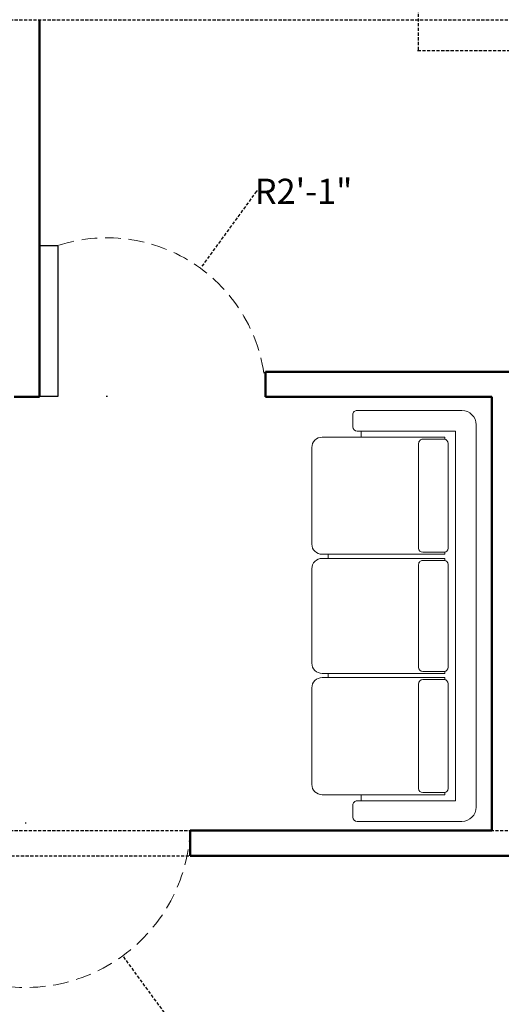
# Model space of a CAD drawing. Units: inches. Extents: x 513 to 1142, y 396 to 927.
# Tile 26 of 31: x 922 to 998, y 614 to 770. Entities that reach past the tile are written whole.
import ezdxf

# ---------------------------------------------------------------- set-up
doc = ezdxf.new("R2010")
doc.units = ezdxf.units.IN
doc.header["$MEASUREMENT"] = 0
doc.linetypes.add('DASHED', pattern=[0.75, 0.5, -0.25])
for name, color, linetype, lineweight in [('A-ANNO-DIMS', 2, 'DASHED', 18), ('A-DOOR', 4, 'Continuous', 25), ('A-DOOR-SWNG', 4, 'DASHED', 13), ('A-WALL', 7, 'Continuous', 50), ('furniture', 92, 'Continuous', 18)]:
    doc.layers.add(name, color=color, linetype=linetype, lineweight=lineweight)
doc.styles.get("Standard").update_dxf_attribs({"font": 'arial.ttf'})
doc.dimstyles.get("Standard").update_dxf_attribs({"dimtxt": 4, "dimasz": 0.18, "dimexe": 0.18, "dimexo": 0.0625, "dimgap": 0.09, "dimtad": 0, "dimtih": 1, "dimtoh": 1, "dimdec": 0, "dimrnd": 6, "dimzin": 0, "dimdsep": 46, "dimlunit": 3, "dimtxsty": 'Standard', "dimcen": 0.09, "dimadec": 0, "dimazin": 0, "dimtfac": 1, "dimtdec": 0, "dimtofl": 0, "dimtmove": 0, "dimatfit": 3, "dimfxl": 1, "dimtolj": 1, "dimtzin": 0, "dimarcsym": 0})

# ---------------------------------------------------------------- blocks, each defined once
blk = doc.blocks.new('A$C06FC73D7')
for p, q in [((1.93, 0.8), (0.07, 0.8)), ((0, 0.73), (0, 0.22)), ((2, 0.22), (2, 0.73)), ((0.1, 0.22), (0.1, 0.7)), ((0.1, 0.7), (1.9, 0.7)), ((1.9, 0.7), (1.9, 0.22)), ((0.13, 0.6479), (0.13, 0.05)), ((0.1404, 0.6479), (0.13, 0.6479)), ((0.14, 0.54), (0.14, 0.6437)), ((0.67, 0.6637), (0.16, 0.6637)), ((0.7, 0.6479), (0.6896, 0.6479)), ((0.69, 0.54), (0.69, 0.6437)), ((0.7, 0.05), (0.7, 0.6479)), ((0.72, 0.05), (0.72, 0.6479)), ((0.7304, 0.6479), (0.72, 0.6479)), ((0.73, 0.54), (0.73, 0.6437)), ((1.25, 0.6637), (0.75, 0.6637)), ((1.28, 0.6479), (1.2696, 0.6479)), ((1.27, 0.54), (1.27, 0.6437)), ((1.28, 0.05), (1.28, 0.6479)), ((1.3, 0.05), (1.3, 0.6479)), ((1.3104, 0.6479), (1.3, 0.6479)), ((1.31, 0.54), (1.31, 0.6437)), ((1.84, 0.6637), (1.33, 0.6637)), ((1.87, 0.6479), (1.86, 0.6479)), ((1.86, 0.54), (1.86, 0.6437)), ((1.87, 0.05), (1.87, 0.6479)), ((0.67, 0.52), (0.16, 0.52)), ((1.25, 0.52), (0.75, 0.52)), ((1.84, 0.52), (1.33, 0.52)), ((0.13, 0.24), (0.1, 0.24)), ((1.9, 0.24), (1.87, 0.24)), ((0.02, 0.2), (0.08, 0.2)), ((1.92, 0.2), (1.98, 0.2)), ((0.72, 0.08), (0.7, 0.08)), ((1.3, 0.08), (1.28, 0.08)), ((0.65, 0), (0.18, 0)), ((1.23, 0), (0.77, 0)), ((1.82, 0), (1.35, 0))]:
    blk.add_line(p, q)
for centre, radius, start, end in [((0.07, 0.73), 0.07, 90, 180), ((1.93, 0.73), 0.07, 0, 90), ((0.16, 0.6437), 0.02, 90, 180), ((0.67, 0.6437), 0.02, 0, 90), ((0.75, 0.6437), 0.02, 90, 180), ((1.25, 0.6437), 0.02, 0, 90), ((1.33, 0.6437), 0.02, 90, 180), ((1.84, 0.6437), 0.02, 0, 90), ((0.16, 0.54), 0.02, 180, 270), ((0.67, 0.54), 0.02, 270, 0), ((0.75, 0.54), 0.02, 180, 270), ((1.25, 0.54), 0.02, 270, 0), ((1.33, 0.54), 0.02, 180, 270), ((1.84, 0.54), 0.02, 270, 0), ((0.02, 0.22), 0.02, 180, 270), ((0.08, 0.22), 0.02, 270, 0), ((1.92, 0.22), 0.02, 180, 270), ((1.98, 0.22), 0.02, 270, 0), ((0.18, 0.05), 0.05, 180, 270), ((0.65, 0.05), 0.05, 270, 0), ((0.77, 0.05), 0.05, 180, 270), ((1.23, 0.05), 0.05, 270, 0), ((1.35, 0.05), 0.05, 180, 270), ((1.82, 0.05), 0.05, 270, 0)]:
    blk.add_arc(centre, radius, start, end)
blk = doc.blocks.new('A$C2BDD4447')
blk.add_blockref('A$C06FC73D7', (0, 0))
blk = doc.blocks.new('DOOR-LEAF-24IN')
blk.add_lwpolyline([(3, 24), (3, 0), (0, 0), (0, 24)], close=True)
blk = doc.blocks.new('*D117')
at = {"layer": 'A-ANNO-DIMS', "color": 0, "lineweight": -2, "transparency": 16777216}
for p, q in [((999.94, 862.98), (985.15, 862.98)), ((985.33, 862.8), (985.33, 816.24)), ((985.33, 765.36), (985.33, 811.92)), ((999.94, 765.18), (985.15, 765.18))]:
    blk.add_line(p, q, dxfattribs=at)
at = {"layer": 'A-ANNO-DIMS', "color": 0, "transparency": 16777216}
for points in [[(985.3, 862.8), (985.36, 862.8), (985.33, 862.98)], [(985.3, 765.36), (985.36, 765.36), (985.33, 765.18)]]:
    blk.add_solid(points, dxfattribs=at)
at = {"layer": 'Defpoints', "color": 0, "transparency": 16777216}
for p in [(1000, 862.98), (985.33, 765.18), (1000, 765.18)]:
    blk.add_point(p, dxfattribs=at)
at = {"layer": 'A-ANNO-DIMS', "color": 0, "transparency": 16777216, "insert": (985.33, 814.08), "char_height": 4, "attachment_point": 5}
blk.add_mtext('\\A1;BED GROUP 8\'-2" TYP.', dxfattribs=at)
blk = doc.blocks.new('*D149')
at = {"layer": 'A-ANNO-DIMS', "color": 0, "lineweight": -2, "transparency": 16777216}
for p, q in [((840.06, 770.16), (1131.58, 770.16)), ((1131.4, 769.98), (1131.4, 707.79)), ((1131.4, 641.34), (1131.4, 703.53)), ((840.06, 641.16), (1131.58, 641.16))]:
    blk.add_line(p, q, dxfattribs=at)
at = {"layer": 'A-ANNO-DIMS', "color": 0, "transparency": 16777216}
for points in [[(1131.37, 769.98), (1131.43, 769.98), (1131.4, 770.16)], [(1131.37, 641.34), (1131.43, 641.34), (1131.4, 641.16)]]:
    blk.add_solid(points, dxfattribs=at)
at = {"layer": 'Defpoints', "color": 0, "transparency": 16777216}
for p in [(840, 770.16), (1131.4, 770.16), (840, 641.16)]:
    blk.add_point(p, dxfattribs=at)
at = {"layer": 'A-ANNO-DIMS', "color": 0, "transparency": 16777216, "insert": (1131.4, 705.66), "char_height": 4, "attachment_point": 5}
blk.add_mtext('\\A1;10\'-9"', dxfattribs=at)
blk = doc.blocks.new('*D173')
at = {"layer": 'A-ANNO-DIMS', "color": 0, "lineweight": -2, "transparency": 16777216}
for p, q in [((904.06, 637.16), (1131.58, 637.16)), ((1131.4, 636.98), (1131.4, 618.76)), ((1131.4, 596.27), (1131.4, 614.49)), ((904.06, 596.09), (1131.58, 596.09))]:
    blk.add_line(p, q, dxfattribs=at)
at = {"layer": 'A-ANNO-DIMS', "color": 0, "transparency": 16777216}
for points in [[(1131.37, 636.98), (1131.43, 636.98), (1131.4, 637.16)], [(1131.37, 596.27), (1131.43, 596.27), (1131.4, 596.09)]]:
    blk.add_solid(points, dxfattribs=at)
at = {"layer": 'Defpoints', "color": 0, "transparency": 16777216}
for p in [(904, 637.16), (1131.4, 637.16), (904, 596.09)]:
    blk.add_point(p, dxfattribs=at)
at = {"layer": 'A-ANNO-DIMS', "color": 0, "transparency": 16777216, "insert": (1131.4, 616.63), "char_height": 4, "attachment_point": 5}
blk.add_mtext('\\A1;3\'-5"', dxfattribs=at)
blk = doc.blocks.new('*D180')
at = {"layer": 'A-ANNO-DIMS', "color": 0, "lineweight": -2, "transparency": 16777216}
for p, q in [((922.75, 642.37), (922.93, 642.37)), ((922.84, 642.28), (922.84, 642.46)), ((947.56, 608.55), (938.4, 621.09)), ((947.74, 608.55), (947.56, 608.55))]:
    blk.add_line(p, q, dxfattribs=at)
at = {"layer": 'A-ANNO-DIMS', "color": 0, "transparency": 16777216}
blk.add_solid([(938.42, 621.11), (938.37, 621.07), (938.29, 621.24)], dxfattribs=at)
at = {"layer": 'Defpoints', "color": 0, "transparency": 16777216}
for p in [(922.84, 642.37), (938.29, 621.24)]:
    blk.add_point(p, dxfattribs=at)
at = {"layer": 'A-ANNO-DIMS', "color": 0, "transparency": 16777216, "insert": (955.06, 608.55), "char_height": 4, "attachment_point": 5}
blk.add_mtext('\\A1;R2\'-2"', dxfattribs=at)
blk = doc.blocks.new('*D181')
at = {"layer": 'A-ANNO-DIMS', "color": 0, "lineweight": -2, "transparency": 16777216}
for p, q in [((959.54, 742.86), (950.73, 730.77)), ((959.72, 742.86), (959.54, 742.86)), ((935.67, 710.24), (935.85, 710.24)), ((935.76, 710.15), (935.76, 710.33))]:
    blk.add_line(p, q, dxfattribs=at)
at = {"layer": 'A-ANNO-DIMS', "color": 0, "transparency": 16777216}
blk.add_solid([(950.71, 730.79), (950.75, 730.76), (950.62, 730.63)], dxfattribs=at)
at = {"layer": 'Defpoints', "color": 0, "transparency": 16777216}
for p in [(950.62, 730.63), (935.76, 710.24)]:
    blk.add_point(p, dxfattribs=at)
at = {"layer": 'A-ANNO-DIMS', "color": 0, "transparency": 16777216, "insert": (967.04, 742.86), "char_height": 4, "attachment_point": 5}
blk.add_mtext('\\A1;R2\'-1"', dxfattribs=at)

msp = doc.modelspace()

# ---------------------------------------------------------------- linework, layer by layer
at = {"layer": 'A-DOOR-SWNG', "ltscale": 5}
for centre, radius, start, end in [((935.76, 710.24), 25.23, 359.8215, 108.0143), ((922.84, 642.37), 26.18, 254.9757, 357.339)]:
    msp.add_arc(centre, radius, start, end, dxfattribs=at)
at = {"layer": 'A-WALL'}
for p, q in [((925, 710.16), (925, 770.16)), ((961, 710.16), (961, 714.16)), ((1001, 714.16), (961, 714.16)), ((925, 710.16), (921, 710.16)), ((997, 710.16), (961, 710.16)), ((997, 641.16), (997, 710.16)), ((949, 637.16), (949, 641.16)), ((949, 641.16), (997, 641.16)), ((949, 637.16), (1001, 637.16))]:
    msp.add_line(p, q, dxfattribs=at)

# ---------------------------------------------------------------- block references
at = {"layer": 'A-DOOR'}
msp.add_blockref('DOOR-LEAF-24IN', (924.96, 710.23), dxfattribs=at)
at = {"layer": 'furniture', "xscale": 32.68979708061804, "yscale": 32.68979708061804, "zscale": 32.68979708061804, "rotation": 270}
msp.add_blockref('A$C2BDD4447', (968.35, 707.99), dxfattribs=at)

# ---------------------------------------------------------------- dimensions: what is measured, and where the dimension line sits
at = {"layer": 'A-ANNO-DIMS'}
dim = msp.add_linear_dim(base=(985.33, 765.18), p1=(1000, 862.98), p2=(1000, 765.18), angle=270, text='BED GROUP <> TYP.', dimstyle='Standard', override={"dimdec": 1, "dimlfac": 1, "dimrnd": 0, "dimzin": 1, "dimdsep": 46, "dimlunit": 4, "dimfrac": 2}, dxfattribs=at)
dim.commit()
dim.dimension.update_dxf_attribs({"geometry": '*D117', "text_midpoint": (985.33, 814.08)})
for base, p1, p2, picture, middle in [((1131.4, 770.16), (840, 641.16), (840, 770.16), '*D149', (1131.4, 705.66)), ((1131.4, 637.16), (904, 596.09), (904, 637.16), '*D173', (1131.4, 616.63))]:
    dim = msp.add_linear_dim(base=base, p1=p1, p2=p2, angle=90, dimstyle='Standard', override={"dimdec": 1, "dimlfac": 1, "dimrnd": 0, "dimzin": 1, "dimdsep": 46, "dimlunit": 4, "dimfrac": 2}, dxfattribs=at)
    dim.commit()
    dim.dimension.update_dxf_attribs({"geometry": picture, "text_midpoint": middle})
for center, mpoint, picture, middle in [((935.76, 710.24), (950.62, 730.63), '*D181', (967.04, 742.86)), ((922.84, 642.37), (938.29, 621.24), '*D180', (955.06, 608.55))]:
    dim = msp.add_radius_dim(center=center, mpoint=mpoint, dimstyle='Standard', override={"dimdec": 1, "dimlfac": 1, "dimrnd": 0, "dimzin": 1, "dimdsep": 46, "dimlunit": 4, "dimfrac": 2}, dxfattribs=at)
    dim.commit()
    dim.dimension.update_dxf_attribs({"geometry": picture, "text_midpoint": middle, "dimtype": 164})

doc.saveas('drawing.dxf')
